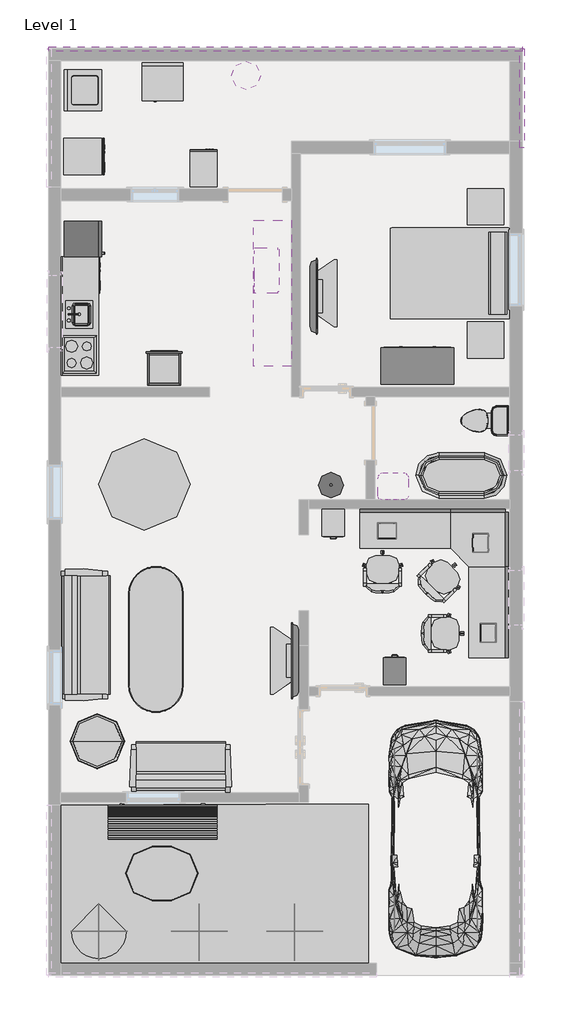
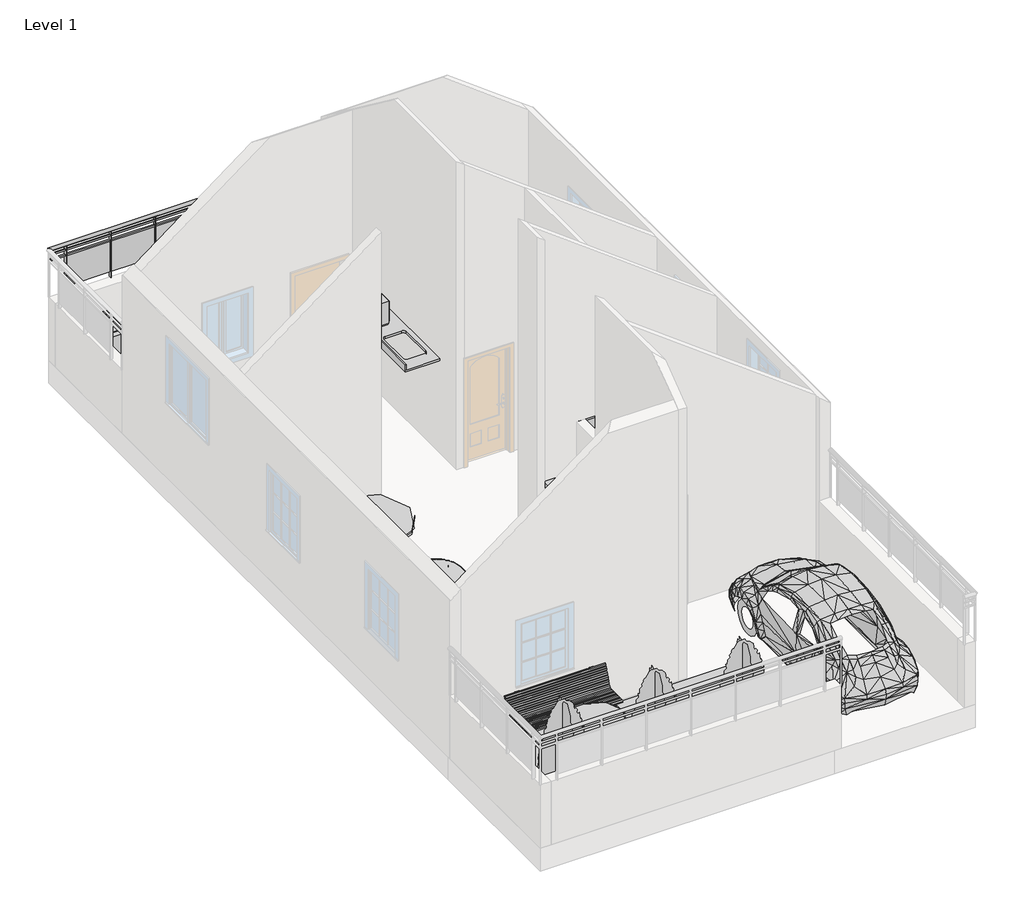
# One storey, part 3 of 3: 22 furniture elements, 15 proxies, 6 flow terminals, 4 geographic elements, 2 railings.
"""IFC4 building model written with IfcOpenShell, lengths in millimetres."""

from ifc_helpers import new_model, si_unit, point, frame, origin, place, context, project, spatial, polyline, ellipse_curve, trimmed, outline, extrude, triangles, transform, mapped, element, save
from ifc_brep_helpers import plane_surface, extruded_surface, advanced_brep
from components import entourage_4c8cfd20, proxy_7e1014cc, proxy_a6faaae8, proxy_45b28599, proxy_19aded4c, proxy_b4d0e45e, kitchenette_medium_kitchenette_medium_844211aa, proxy_8a8d5ab2, proxy_8b8c2dc4, rpc_beetle_rpc_beetle_3ce7ba48, proxy_c523a7b7, proxy_718fa39f, flow_terminal_871c2e40, flow_terminal_d49f872f, flow_terminal_62a433f7, toilet_domestic_3d_toilet_domestic_3d_f7549cf7, toilet_domestic_3d_toilet_domestic_3d_183bbd19, flow_terminal_b374fae2, furniture_e1791683, furniture_bb55ed6b, furniture_b1353b55, chair_executive_chair_executive_8d69e98c, furniture_22cae41e, furniture_c6510c7c, furniture_9fa109b2, furniture_ad7727fe, furniture_aff9b2fb, furniture_fdf74506, tv_stand_tv_stand_6ce107e5, furniture_be1c6672, furniture_e05f6f82, furniture_bbcc68ce, furniture_5bc9ed15, furniture_c80d6d9c, furniture_45e3acac, geographic_element_235d1464, rpc_tree_conifer_chinese_juniper_7_1b9786cd

model = new_model("IFC4")

# Units and contexts
model_context = context("Model", 3, world=origin())
ifc_project = project(units=[si_unit("LENGTHUNIT", "METRE", prefix="MILLI")], contexts=[model_context])

# Site, building, storey
site = spatial("IfcSite", under=ifc_project)
building = spatial("IfcBuilding", under=site)
storey = spatial("IfcBuildingStorey", under=building, Name="Level 1", Elevation=0.0)

# Proxies
placement = place(None, origin())
element("IfcBuildingElementProxy", 1, Name="Building Element Proxy", at=placement, inside=storey, context=model_context, shape_type="Tessellation", body=[
    triangles([(-7981.8122177, -789.0605576, 0.0), (-2825.6124115, -763.6605818, 0.0), (-2825.6124115, -3430.6606544, 0.0), (-7981.8122177, -3430.6606544, 0.0)], [[1, 4, 3], [3, 2, 1]], closed=False),
])
entourage_shape = entourage_4c8cfd20(model_context)
element("IfcBuildingElementProxy", 2, Name="Entourage", at=placement, inside=storey, context=model_context, shape_type="MappedRepresentation", body=[
    mapped(entourage_shape, transform((-793.6124913, 2092.734912, 762.0), x_axis=(0.0, -1.0000000000000004, 0.0), y_axis=(1.0000000000000004, 0.0, 0.0), z_axis=(0.0, 0.0, 1.0))),
])
element("IfcBuildingElementProxy", 3, Name="Entourage", at=placement, inside=storey, context=model_context, shape_type="MappedRepresentation", body=[
    mapped(entourage_shape, transform((-2522.3706258, 3833.7394299, 762.0), x_axis=(1.0000000000000004, 0.0, 0.0), y_axis=(0.0, 1.0000000000000004, 0.0), z_axis=(0.0, 0.0, 1.0))),
])
element("IfcBuildingElementProxy", 4, Name="Entourage", at=placement, inside=storey, context=model_context, shape_type="MappedRepresentation", body=[
    mapped(entourage_shape, transform((-920.6124913, 3598.218512, 762.0), x_axis=(0.0, -1.0000000000000002, 0.0), y_axis=(1.0000000000000002, 0.0, 0.0), z_axis=(0.0, 0.0, 1.0))),
])
proxy_shape = proxy_7e1014cc(model_context)
element("IfcBuildingElementProxy", 5, Name="18\" x 24\" x 34 1/2\"", ObjectType="18\" x 24\" x 34 1/2\"", at=placement, inside=storey, context=model_context, shape_type="MappedRepresentation", body=[
    mapped(proxy_shape, transform((-5288.0950228, 10123.1639947, 0.0), x_axis=(-1.0, 0.0, 0.0), y_axis=(0.0, -1.0, 0.0), z_axis=(0.0, 0.0, 1.0))),
])
proxy_2_shape = proxy_a6faaae8(model_context)
element("IfcBuildingElementProxy", 6, Name="Cook Top-4 Unit2 : 22\" x 20\"", ObjectType="Cook Top-4 Unit2 : 22\" x 20\"", at=placement, inside=storey, context=model_context, shape_type="MappedRepresentation", body=[
    mapped(proxy_2_shape, transform((-7677.0124913, 6745.2144299, 0.0), x_axis=(0.0, 0.9999999999999999, 0.0), y_axis=(-0.9999999999999999, 0.0, 0.0), z_axis=(0.0, 0.0, 1.0))),
])
proxy_3_shape = proxy_45b28599(model_context)
element("IfcBuildingElementProxy", 7, Name="Dishwasher : 24\" x 24\" x 34\"", ObjectType="Dishwasher : 24\" x 24\" x 34\"", at=placement, inside=storey, context=model_context, shape_type="MappedRepresentation", body=[
    mapped(proxy_3_shape, transform((-7385.1629265, 7696.3969614, 0.0), x_axis=(0.0, 0.9999999999999999, 0.0), y_axis=(-0.9999999999999999, 0.0, 0.0), z_axis=(0.0, 0.0, 1.0))),
])
proxy_4_shape = proxy_19aded4c(model_context)
element("IfcBuildingElementProxy", 8, Name="Dishwasher : 24\" x 26 1/4\" x 34 1/2\"", ObjectType="Dishwasher : 24\" x 26 1/4\" x 34 1/2\"", at=placement, inside=storey, context=model_context, shape_type="MappedRepresentation", body=[
    mapped(proxy_4_shape, transform((-7308.9629265, 9674.4219614, 0.0), x_axis=(0.0, 1.0000000000000002, 0.0), y_axis=(-1.0000000000000002, 0.0, 0.0), z_axis=(0.0, 0.0, 1.0))),
])
proxy_5_shape = proxy_b4d0e45e(model_context)
element("IfcBuildingElementProxy", 9, Name="Dryer : 27\" x 25\" x 35\"", ObjectType="Dryer : 27\" x 25\" x 35\"", at=placement, inside=storey, context=model_context, shape_type="MappedRepresentation", body=[
    mapped(proxy_5_shape, transform((-6661.0124913, 10996.5394299, 0.0), x_axis=(1.0000000000000004, 0.0, 0.0), y_axis=(0.0, 1.0000000000000004, 0.0), z_axis=(0.0, 0.0, 1.0))),
])
kitchenette_medium_kitchenette_medium_shape = kitchenette_medium_kitchenette_medium_844211aa(model_context)
element("IfcBuildingElementProxy", 10, Name="Kitchenette - Medium : Kitchenette - Medium", ObjectType="Kitchenette - Medium : Kitchenette - Medium", at=placement, inside=storey, context=model_context, shape_type="MappedRepresentation", body=[
    mapped(kitchenette_medium_kitchenette_medium_shape, transform((-7981.8124913, 7069.376725, 0.0), x_axis=(0.0, 0.9999999999999999, 0.0), y_axis=(-0.9999999999999999, 0.0, 0.0), z_axis=(0.0, 0.0, 1.0))),
])
proxy_6_shape = proxy_8a8d5ab2(model_context)
element("IfcBuildingElementProxy", 11, Name="Microwave : 30\" x 16\" x 18\"", ObjectType="Microwave : 30\" x 16\" x 18\"", at=placement, inside=storey, context=model_context, shape_type="MappedRepresentation", body=[
    mapped(proxy_6_shape, transform((-4180.6819855, 8652.0323072, 914.4), x_axis=(0.0, -1.0000000000000004, 0.0), y_axis=(1.0000000000000004, 0.0, 0.0), z_axis=(0.0, 0.0, 1.0))),
])
proxy_7_shape = proxy_8b8c2dc4(model_context)
element("IfcBuildingElementProxy", 12, Name="Oven Double-Built-in : 21 1/2\" x 39 1/4\" x 21\"", ObjectType="Oven Double-Built-in : 21 1/2\" x 39 1/4\" x 21\"", at=placement, inside=storey, context=model_context, shape_type="MappedRepresentation", body=[
    mapped(proxy_7_shape, transform((-6289.7874186, 6644.9802888, 0.0), x_axis=(-1.0000000000000004, 0.0, 0.0), y_axis=(0.0, -1.0000000000000004, 0.0), z_axis=(0.0, 0.0, 1.0))),
])
rpc_beetle_rpc_beetle_shape = rpc_beetle_rpc_beetle_3ce7ba48(model_context)
element("IfcBuildingElementProxy", 13, Name="RPC Beetle : RPC Beetle", ObjectType="RPC Beetle : RPC Beetle", at=placement, inside=storey, context=model_context, shape_type="MappedRepresentation", body=[
    mapped(rpc_beetle_rpc_beetle_shape, transform((-1708.0124913, -2589.2855701, 0.0), x_axis=(1.0, 0.0, 0.0), y_axis=(0.0, 1.0, 0.0), z_axis=(0.0, 0.0, 1.0))),
])
proxy_8_shape = proxy_c523a7b7(model_context)
element("IfcBuildingElementProxy", 14, Name="Refrigerator : 24\" x 25\" LH", ObjectType="Refrigerator : 24\" x 25\" LH", at=placement, inside=storey, context=model_context, shape_type="MappedRepresentation", body=[
    mapped(proxy_8_shape, transform((-7631.3635198, 8681.9644299, 0.0), x_axis=(0.0, 0.9999999999999999, 0.0), y_axis=(-0.9999999999999999, 0.0, 0.0), z_axis=(0.0, 0.0, 1.0))),
])
proxy_9_shape = proxy_718fa39f(model_context)
element("IfcBuildingElementProxy", 15, Name="Washer : 27\" x 25\" x 35\"", ObjectType="Washer : 27\" x 25\" x 35\"", at=placement, inside=storey, context=model_context, shape_type="MappedRepresentation", body=[
    mapped(proxy_9_shape, transform((-7334.3629265, 10744.3969614, 0.0), x_axis=(0.0, 1.0000000000000027, 0.0), y_axis=(-1.0000000000000027, 0.0, 0.0), z_axis=(0.0, 0.0, 1.0))),
])

# Flow terminals
flow_terminal_shape = flow_terminal_871c2e40(model_context)
element("IfcFlowTerminal", 16, ObjectType="Sink Kitchen-Island : 18\" x 18\"", at=placement, inside=storey, context=model_context, shape_type="MappedRepresentation", body=[
    mapped(flow_terminal_shape, transform((-7674.6670902, 7402.6251893, -14.4), x_axis=(0.0, 0.9999999999999999, 0.0), y_axis=(-0.9999999999999999, 0.0, 0.0), z_axis=(0.0, 0.0, 1.0))),
])
flow_terminal_2_shape = flow_terminal_d49f872f(model_context)
element("IfcFlowTerminal", 17, ObjectType="Sink Vanity-Round : 19\" x 19\"", at=placement, inside=storey, context=model_context, shape_type="MappedRepresentation", body=[
    mapped(flow_terminal_2_shape, transform((-4979.6642319, 11328.3270307, 914.4), x_axis=(1.0, 0.0, 0.0), y_axis=(0.0, 1.0, 0.0), z_axis=(0.0, 0.0, 1.0))),
])
element("IfcFlowTerminal", 18, ObjectType="Sink Vanity-Round : 19\" x 19\"", at=placement, inside=storey, context=model_context, shape_type="MappedRepresentation", body=[
    mapped(flow_terminal_2_shape, transform((-3363.9607507, 4648.8362448, 609.6), x_axis=(-1.0, 0.0, 0.0), y_axis=(0.0, -1.0, 0.0), z_axis=(0.0, 0.0, 1.0))),
])
flow_terminal_3_shape = flow_terminal_62a433f7(model_context)
element("IfcFlowTerminal", 19, ObjectType="Sink Vanity-Square : 20\" x 18\"", at=placement, inside=storey, context=model_context, shape_type="MappedRepresentation", body=[
    mapped(flow_terminal_3_shape, transform((-2403.5232507, 4496.484831, 914.4), x_axis=(-1.0, 0.0, 0.0), y_axis=(0.0, -1.0, 0.0), z_axis=(0.0, 0.0, 1.0))),
])
toilet_domestic_3d_toilet_domestic_3d_shape = toilet_domestic_3d_toilet_domestic_3d_f7549cf7(model_context)
toilet_domestic_3d_toilet_domestic_3d_2_shape = toilet_domestic_3d_toilet_domestic_3d_183bbd19(model_context)
element("IfcFlowTerminal", 20, ObjectType="Toilet-Domestic-3D : Toilet-Domestic-3D", at=placement, inside=storey, context=model_context, shape_type="MappedRepresentation", body=[
    mapped(toilet_domestic_3d_toilet_domestic_3d_shape, transform((-983.5085187, 5640.3144299, 0.0), x_axis=(0.0, -1.0, 0.0), y_axis=(1.0, 0.0, 0.0), z_axis=(0.0, 0.0, 1.0))),
    mapped(toilet_domestic_3d_toilet_domestic_3d_2_shape, transform((-983.5085187, 5640.3144299, 0.0), x_axis=(0.0, -1.0, 0.0), y_axis=(1.0, 0.0, 0.0), z_axis=(0.0, 0.0, 1.0))),
])
flow_terminal_4_shape = flow_terminal_b374fae2(model_context)
element("IfcFlowTerminal", 21, ObjectType="Tub-Free Standing-3D : 30\" x 60\"", at=placement, inside=storey, context=model_context, shape_type="MappedRepresentation", body=[
    mapped(flow_terminal_4_shape, transform((-1276.2124913, 4725.9144299, 0.0), x_axis=(0.0, -1.0000000000000002, 0.0), y_axis=(1.0000000000000002, 0.0, 0.0), z_axis=(0.0, 0.0, 1.0))),
])

# Furniture
furniture_shape = furniture_e1791683(model_context)
element("IfcFurniture", 22, ObjectType="Bed-Standard.0001 : Queen 60\" x 79\"", at=placement, inside=storey, context=model_context, shape_type="MappedRepresentation", body=[
    mapped(furniture_shape, transform((-1421.1174093, 8375.6029545, 0.0), x_axis=(0.0, -1.0, 0.0), y_axis=(1.0, 0.0, 0.0), z_axis=(0.0, 0.0, 1.0))),
])
furniture_2_shape = furniture_bb55ed6b(model_context)
element("IfcFurniture", 23, ObjectType="Cabinet-File 2 Drawer : 15\" x 18\"", at=placement, inside=storey, context=model_context, shape_type="MappedRepresentation", body=[
    mapped(furniture_2_shape, transform((-3294.6160443, 4077.47373, 0.0), x_axis=(1.0, 0.0, 0.0), y_axis=(0.0, 1.0, 0.0), z_axis=(0.0, 0.0, 1.0))),
])
furniture_3_shape = furniture_b1353b55(model_context)
element("IfcFurniture", 24, ObjectType="Cabinet-File 4 Drawer : 15\" x 18\"", at=placement, inside=storey, context=model_context, shape_type="MappedRepresentation", body=[
    mapped(furniture_3_shape, transform((-2521.7089384, 1307.1801298, 0.0), x_axis=(-1.0, 0.0, 0.0), y_axis=(0.0, -1.0, 0.0), z_axis=(0.0, 0.0, 1.0))),
])
chair_executive_chair_executive_shape = chair_executive_chair_executive_8d69e98c(model_context)
element("IfcFurniture", 25, ObjectType="Chair-Executive : Chair-Executive", at=placement, inside=storey, context=model_context, shape_type="MappedRepresentation", body=[
    mapped(chair_executive_chair_executive_shape, transform((-2738.003311, 3103.5935283, 0.0), x_axis=(1.0, 0.0, 0.0), y_axis=(0.0, 1.0, 0.0), z_axis=(0.0, 0.0, 1.0))),
])
element("IfcFurniture", 26, ObjectType="Chair-Executive : Chair-Executive", at=placement, inside=storey, context=model_context, shape_type="MappedRepresentation", body=[
    mapped(chair_executive_chair_executive_shape, transform((-1599.958393, 2222.1302496, 0.0), x_axis=(0.0, -1.0000000000000004, 0.0), y_axis=(1.0000000000000004, 0.0, 0.0), z_axis=(0.0, 0.0, 1.0))),
])
element("IfcFurniture", 27, ObjectType="Chair-Executive : Chair-Executive", at=placement, inside=storey, context=model_context, shape_type="MappedRepresentation", body=[
    mapped(chair_executive_chair_executive_shape, transform((-1730.3328147, 3085.013219, 0.0), x_axis=(0.7071067811865468, -0.7071067811865482, 0.0), y_axis=(0.7071067811865482, 0.7071067811865468, 0.0), z_axis=(0.0, 0.0, 1.0))),
])
furniture_4_shape = furniture_22cae41e(model_context)
element("IfcFurniture", 28, ObjectType="Counter Top w Sink Hole : 24\" Depth", at=placement, inside=storey, context=model_context, shape_type="MappedRepresentation", body=[
    mapped(furniture_4_shape, transform((-4756.0124913, 7755.176725, 914.4), x_axis=(0.0, 1.0, 0.0), y_axis=(-1.0, 0.0, 0.0), z_axis=(0.0, 0.0, 1.0))),
])
furniture_5_shape = furniture_c6510c7c(model_context)
element("IfcFurniture", 29, ObjectType="Counter Top w Sink Hole : 24\" Depth", at=placement, inside=storey, context=model_context, shape_type="MappedRepresentation", body=[
    mapped(furniture_5_shape, transform((-7981.8124913, 7602.776725, -14.4), x_axis=(0.0, 0.9999999999999999, 0.0), y_axis=(-0.9999999999999999, 0.0, 0.0), z_axis=(0.0, 0.0, 1.0))),
])
furniture_6_shape = furniture_9fa109b2(model_context)
element("IfcFurniture", 30, ObjectType="Dresser : 48\" x 72\" x 24\"", at=placement, inside=storey, context=model_context, shape_type="MappedRepresentation", body=[
    mapped(furniture_6_shape, transform((-2282.0057511, 6191.5514758, 0.0), x_axis=(-1.0000000000000004, 0.0, 0.0), y_axis=(0.0, -1.0000000000000004, 0.0), z_axis=(0.0, 0.0, 1.0))),
])
furniture_7_shape = furniture_ad7727fe(model_context)
element("IfcFurniture", 31, ObjectType="Sofa-Pensi : 65\"", at=placement, inside=storey, context=model_context, shape_type="MappedRepresentation", body=[
    mapped(furniture_7_shape, transform((-5696.6062413, 126.224266, 0.0), x_axis=(-1.0, 0.0, 0.0), y_axis=(0.0, -1.0, 0.0), z_axis=(0.0, 0.0, 1.0))),
])
furniture_8_shape = furniture_aff9b2fb(model_context)
element("IfcFurniture", 32, ObjectType="Sofa-Pensi : 84\"", at=placement, inside=storey, context=model_context, shape_type="MappedRepresentation", body=[
    mapped(furniture_8_shape, transform((-7298.3026552, 1780.3081799, 0.0), x_axis=(0.0, 1.0, 0.0), y_axis=(-1.0, 0.0, 0.0), z_axis=(0.0, 0.0, 1.0))),
])
furniture_9_shape = furniture_fdf74506(model_context)
element("IfcFurniture", 33, ObjectType="TV - Flat Screen : 50\"", at=placement, inside=storey, context=model_context, shape_type="MappedRepresentation", body=[
    mapped(furniture_9_shape, transform((-3757.6738677, 7723.883944, 914.4), x_axis=(0.0, 1.0000000000000002, 0.0), y_axis=(-1.0000000000000002, 0.0, 0.0), z_axis=(0.0, 0.0, 1.0))),
])
element("IfcFurniture", 34, ObjectType="TV - Flat Screen : 50\"", at=placement, inside=storey, context=model_context, shape_type="MappedRepresentation", body=[
    mapped(furniture_9_shape, transform((-4052.551115, 1621.6081753, 914.4), x_axis=(0.0, -1.0000000000000007, 0.0), y_axis=(1.0000000000000007, 0.0, 0.0), z_axis=(0.0, 0.0, 1.0))),
])
tv_stand_tv_stand_shape = tv_stand_tv_stand_6ce107e5(model_context)
element("IfcFurniture", 35, ObjectType="TV Stand : TV Stand", at=placement, inside=storey, context=model_context, shape_type="MappedRepresentation", body=[
    mapped(tv_stand_tv_stand_shape, transform((-3816.2124913, 7648.7264278, 0.0), x_axis=(0.0, 1.0, 0.0), y_axis=(-1.0, 0.0, 0.0), z_axis=(0.0, 0.0, 1.0))),
])
element("IfcFurniture", 36, ObjectType="TV Stand : TV Stand", at=placement, inside=storey, context=model_context, shape_type="MappedRepresentation", body=[
    mapped(tv_stand_tv_stand_shape, transform((-4019.4124913, 1752.302432, 0.0), x_axis=(0.0, -1.0000000000000004, 0.0), y_axis=(1.0000000000000004, 0.0, 0.0), z_axis=(0.0, 0.0, 1.0))),
])
furniture_10_shape = furniture_be1c6672(model_context)
element("IfcFurniture", 37, ObjectType="Table-Dining Oval : 36\" x 48\"", at=placement, inside=storey, context=model_context, shape_type="MappedRepresentation", body=[
    mapped(furniture_10_shape, transform((-5889.7477591, -1573.9622094, 0.0), x_axis=(1.0, 0.0, 0.0), y_axis=(0.0, 1.0, 0.0), z_axis=(0.0, 0.0, 1.0))),
])
furniture_11_shape = furniture_e05f6f82(model_context)
element("IfcFurniture", 38, ObjectType="Table-Dining Oval : 36\" x 96\" Laminate Top", at=placement, inside=storey, context=model_context, shape_type="MappedRepresentation", body=[
    mapped(furniture_11_shape, transform((-6748.2575678, 2384.534102, 0.0), x_axis=(0.0, 1.0000000000000002, 0.0), y_axis=(-1.0000000000000002, 0.0, 0.0), z_axis=(0.0, 0.0, 1.0))),
])
furniture_12_shape = furniture_bbcc68ce(model_context)
element("IfcFurniture", 39, ObjectType="Table-Dining Round w Chairs : 60\" Diameter", at=placement, inside=storey, context=model_context, shape_type="MappedRepresentation", body=[
    mapped(furniture_12_shape, transform((-6688.4944585, 4758.3931184, 0.0), x_axis=(1.0, 0.0, 0.0), y_axis=(0.0, 1.0, 0.0), z_axis=(0.0, 0.0, 1.0))),
])
furniture_13_shape = furniture_5bc9ed15(model_context)
element("IfcFurniture", 40, ObjectType="Table-Night Stand : 24\" x 24\" x 30\"", at=placement, inside=storey, context=model_context, shape_type="MappedRepresentation", body=[
    mapped(furniture_13_shape, transform((-1178.3461216, 8913.7394299, 0.0), x_axis=(1.0, 0.0, 0.0), y_axis=(0.0, 1.0, 0.0), z_axis=(0.0, 0.0, 1.0))),
])
element("IfcFurniture", 41, ObjectType="Table-Night Stand : 24\" x 24\" x 30\"", at=placement, inside=storey, context=model_context, shape_type="MappedRepresentation", body=[
    mapped(furniture_13_shape, transform((-1178.3461216, 6681.7144299, 0.0), x_axis=(1.0, 0.0, 0.0), y_axis=(0.0, 1.0, 0.0), z_axis=(0.0, 0.0, 1.0))),
])
furniture_14_shape = furniture_c80d6d9c(model_context)
element("IfcFurniture", 42, ObjectType="Table-Round : 36\" Diameter", at=placement, inside=storey, context=model_context, shape_type="MappedRepresentation", body=[
    mapped(furniture_14_shape, transform((-7372.2124913, 277.7394299, 0.0), x_axis=(1.0, 0.0, 0.0), y_axis=(0.0, 1.0, 0.0), z_axis=(0.0, 0.0, 1.0))),
])
furniture_15_shape = furniture_45e3acac(model_context)
element("IfcFurniture", 43, ObjectType="Work Station Cubicle : 96\" x 96\"", at=placement, inside=storey, context=model_context, shape_type="MappedRepresentation", body=[
    mapped(furniture_15_shape, transform((6.2105163, 4032.2076777, 0.0), x_axis=(0.0, -1.0000000000000004, 0.0), y_axis=(1.0000000000000004, 0.0, 0.0), z_axis=(0.0, 0.0, 1.0))),
])

# Geographic elements
geographic_element_shape = geographic_element_235d1464(model_context)
element("IfcGeographicElement", 44, ObjectType="Park Bench : 72\"", at=placement, inside=storey, context=model_context, shape_type="MappedRepresentation", body=[
    mapped(geographic_element_shape, transform((-6280.0124913, -1043.0605701, 0.0), x_axis=(1.0, 0.0, 0.0), y_axis=(0.0, 1.0, 0.0), z_axis=(0.0, 0.0, 1.0))),
])
rpc_tree_conifer_chinese_juniper_7_shape = rpc_tree_conifer_chinese_juniper_7_1b9786cd(model_context)
element("IfcGeographicElement", 45, ObjectType="RPC Tree - Conifer : Chinese Juniper - 7'", at=placement, inside=storey, context=model_context, shape_type="MappedRepresentation", body=[
    mapped(rpc_tree_conifer_chinese_juniper_7_shape, transform((-7347.0091624, -2897.2605701, 0.0), x_axis=(1.0, 0.0, 0.0), y_axis=(0.0, 1.0, 0.0), z_axis=(0.0, 0.0, 1.0))),
])
element("IfcGeographicElement", 46, ObjectType="RPC Tree - Conifer : Chinese Juniper - 7'", at=placement, inside=storey, context=model_context, shape_type="MappedRepresentation", body=[
    mapped(rpc_tree_conifer_chinese_juniper_7_shape, transform((-5670.6091624, -2897.2605701, 0.0), x_axis=(1.0, 0.0, 0.0), y_axis=(0.0, 1.0, 0.0), z_axis=(0.0, 0.0, 1.0))),
])
element("IfcGeographicElement", 47, ObjectType="RPC Tree - Conifer : Chinese Juniper - 7'", at=placement, inside=storey, context=model_context, shape_type="MappedRepresentation", body=[
    mapped(rpc_tree_conifer_chinese_juniper_7_shape, transform((-4070.4091624, -2897.2605701, 0.0), x_axis=(1.0, 0.0, 0.0), y_axis=(0.0, 1.0, 0.0), z_axis=(0.0, 0.0, 1.0))),
])

# Railings
element("IfcRailing", 48, ObjectType="Glass Panel - Bottom Fill", at=placement, inside=storey, context=model_context, shape_type="SolidModel", body=[
    advanced_brep(
    [(-8185.0124913, 11898.2394299, 2133.6), (-8185.0124913, 11822.0394299, 2133.6), (-260.2124913, 11898.2394299, 2133.6), (-260.2124913, 11822.0394299, 2133.6)],
    [
        (0, 1, ellipse_curve(frame((-8185.0124913, 11860.1394299, 2133.6), z_axis=(-1.0, 0.0, 0.0), x_axis=(0.0, -1.0, 0.0)), 38.1, 28.575)),
        (1, 0, ellipse_curve(frame((-8185.0124913, 11860.1394299, 2133.6), z_axis=(-1.0, 0.0, 0.0), x_axis=(0.0, -1.0, 0.0)), 38.1, 28.575)),
        (2, 3, ellipse_curve(frame((-260.2124913, 11860.1394299, 2133.6), z_axis=(1.0, 0.0, 0.0), x_axis=(0.0, -1.0, 0.0)), 38.1, 28.575)),
        (3, 2, ellipse_curve(frame((-260.2124913, 11860.1394299, 2133.6), z_axis=(1.0, 0.0, 0.0), x_axis=(0.0, -1.0, 0.0)), 38.1, 28.575)),
        (0, 2),
        (3, 1),
    ],
    [
        plane_surface(frame((-8185.0124913, 11860.1394299, 2133.6), z_axis=(-1.0, 0.0, 0.0), x_axis=(0.0, 1.0, 0.0))),
        plane_surface(frame((-260.2124913, 11860.1394299, 2133.6), z_axis=(1.0, 0.0, 0.0), x_axis=(0.0, 1.0, 0.0))),
        extruded_surface(trimmed(ellipse_curve(frame((-260.2124913, 11860.1394299, 2133.6), z_axis=(-1.0, 0.0, 0.0), x_axis=(0.0, -1.0, 0.0)), 38.1, 28.575), [point((-260.2124913, 11898.2394299, 2133.6))], [point((-260.2124913, 11822.0394299, 2133.6))], True, "CARTESIAN"), (-7924.8, 0.0, 0.0), 7924.8),
        extruded_surface(trimmed(ellipse_curve(frame((-260.2124913, 11860.1394299, 2133.6), z_axis=(-1.0, 0.0, 0.0), x_axis=(0.0, -1.0, 0.0)), 38.1, 28.575), [point((-260.2124913, 11822.0394299, 2133.6))], [point((-260.2124913, 11898.2394299, 2133.6))], True, "CARTESIAN"), (-7924.8, 0.0, 0.0), 7924.8),
    ],
    [
        (0, [[1, 2]]),
        (1, [[3, 4]]),
        (2, [[-1, 5, -4, 6]]),
        (3, [[-2, -6, -3, -5]]),
    ],
),
    extrude(outline(polyline([(-8185.0124913, 11847.4394299), (-8185.0124913, 11872.8394299), (-260.2124913, 11872.8394299), (-260.2124913, 11847.4394299), (-8185.0124913, 11847.4394299)])), frame((0.0, 0.0, 2019.3), z_axis=(0.0, 0.0, 1.0), x_axis=(1.0, 0.0, 0.0)), (0.0, 0.0, 1.0), 25.4),
    extrude(outline(polyline([(-8185.0124913, 11847.4394299), (-8185.0124913, 11872.8394299), (-260.2124913, 11872.8394299), (-260.2124913, 11847.4394299), (-8185.0124913, 11847.4394299)])), frame((0.0, 0.0, 1917.7), z_axis=(0.0, 0.0, 1.0), x_axis=(1.0, 0.0, 0.0)), (0.0, 0.0, 1.0), 25.4),
    extrude(outline(polyline([(-571.3624913, 11834.7394299), (-571.3624913, 11885.5394299), (-558.6624913, 11885.5394299), (-558.6624913, 11834.7394299), (-571.3624913, 11834.7394299)])), frame((0.0, 0.0, 1219.2), z_axis=(0.0, 0.0, 1.0), x_axis=(1.0, 0.0, 0.0)), (0.0, 0.0, 1.0), 885.6788223),
    extrude(outline(polyline([(-1377.8124913, 11866.6745869), (-565.0124913, 11866.6745869), (-565.0124913, 11860.3245869), (-1377.8124913, 11860.3245869), (-1377.8124913, 11866.6745869)])), frame((0.0, 0.0, 1320.8), z_axis=(0.0, 0.0, 1.0), x_axis=(1.0, 0.0, 0.0)), (0.0, 0.0, 1.0), 596.9),
    extrude(outline(polyline([(-1384.1624913, 11834.7394299), (-1384.1624913, 11885.5394299), (-1371.4624913, 11885.5394299), (-1371.4624913, 11834.7394299), (-1384.1624913, 11834.7394299)])), frame((0.0, 0.0, 1219.2), z_axis=(0.0, 0.0, 1.0), x_axis=(1.0, 0.0, 0.0)), (0.0, 0.0, 1.0), 885.6788223),
    extrude(outline(polyline([(-2190.6124913, 11866.6745869), (-1377.8124913, 11866.6745869), (-1377.8124913, 11860.3245869), (-2190.6124913, 11860.3245869), (-2190.6124913, 11866.6745869)])), frame((0.0, 0.0, 1320.8), z_axis=(0.0, 0.0, 1.0), x_axis=(1.0, 0.0, 0.0)), (0.0, 0.0, 1.0), 596.9),
    extrude(outline(polyline([(-2196.9624913, 11834.7394299), (-2196.9624913, 11885.5394299), (-2184.2624913, 11885.5394299), (-2184.2624913, 11834.7394299), (-2196.9624913, 11834.7394299)])), frame((0.0, 0.0, 1219.2), z_axis=(0.0, 0.0, 1.0), x_axis=(1.0, 0.0, 0.0)), (0.0, 0.0, 1.0), 885.6788223),
    extrude(outline(polyline([(-3003.4124913, 11866.6745869), (-2190.6124913, 11866.6745869), (-2190.6124913, 11860.3245869), (-3003.4124913, 11860.3245869), (-3003.4124913, 11866.6745869)])), frame((0.0, 0.0, 1320.8), z_axis=(0.0, 0.0, 1.0), x_axis=(1.0, 0.0, 0.0)), (0.0, 0.0, 1.0), 596.9),
    extrude(outline(polyline([(-3009.7624913, 11834.7394299), (-3009.7624913, 11885.5394299), (-2997.0624913, 11885.5394299), (-2997.0624913, 11834.7394299), (-3009.7624913, 11834.7394299)])), frame((0.0, 0.0, 1219.2), z_axis=(0.0, 0.0, 1.0), x_axis=(1.0, 0.0, 0.0)), (0.0, 0.0, 1.0), 885.6788223),
    extrude(outline(polyline([(-3816.2124913, 11866.6745869), (-3003.4124913, 11866.6745869), (-3003.4124913, 11860.3245869), (-3816.2124913, 11860.3245869), (-3816.2124913, 11866.6745869)])), frame((0.0, 0.0, 1320.8), z_axis=(0.0, 0.0, 1.0), x_axis=(1.0, 0.0, 0.0)), (0.0, 0.0, 1.0), 596.9),
    extrude(outline(polyline([(-3822.5624913, 11834.7394299), (-3822.5624913, 11885.5394299), (-3809.8624913, 11885.5394299), (-3809.8624913, 11834.7394299), (-3822.5624913, 11834.7394299)])), frame((0.0, 0.0, 1219.2), z_axis=(0.0, 0.0, 1.0), x_axis=(1.0, 0.0, 0.0)), (0.0, 0.0, 1.0), 885.6788223),
    extrude(outline(polyline([(-4629.0124913, 11866.6745869), (-3816.2124913, 11866.6745869), (-3816.2124913, 11860.3245869), (-4629.0124913, 11860.3245869), (-4629.0124913, 11866.6745869)])), frame((0.0, 0.0, 1320.8), z_axis=(0.0, 0.0, 1.0), x_axis=(1.0, 0.0, 0.0)), (0.0, 0.0, 1.0), 596.9),
    extrude(outline(polyline([(-4635.3624913, 11834.7394299), (-4635.3624913, 11885.5394299), (-4622.6624913, 11885.5394299), (-4622.6624913, 11834.7394299), (-4635.3624913, 11834.7394299)])), frame((0.0, 0.0, 1219.2), z_axis=(0.0, 0.0, 1.0), x_axis=(1.0, 0.0, 0.0)), (0.0, 0.0, 1.0), 885.6788223),
    extrude(outline(polyline([(-5441.8124913, 11866.6745869), (-4629.0124913, 11866.6745869), (-4629.0124913, 11860.3245869), (-5441.8124913, 11860.3245869), (-5441.8124913, 11866.6745869)])), frame((0.0, 0.0, 1320.8), z_axis=(0.0, 0.0, 1.0), x_axis=(1.0, 0.0, 0.0)), (0.0, 0.0, 1.0), 596.9),
    extrude(outline(polyline([(-5448.1624913, 11834.7394299), (-5448.1624913, 11885.5394299), (-5435.4624913, 11885.5394299), (-5435.4624913, 11834.7394299), (-5448.1624913, 11834.7394299)])), frame((0.0, 0.0, 1219.2), z_axis=(0.0, 0.0, 1.0), x_axis=(1.0, 0.0, 0.0)), (0.0, 0.0, 1.0), 885.6788223),
    extrude(outline(polyline([(-6254.6124913, 11866.6745869), (-5441.8124913, 11866.6745869), (-5441.8124913, 11860.3245869), (-6254.6124913, 11860.3245869), (-6254.6124913, 11866.6745869)])), frame((0.0, 0.0, 1320.8), z_axis=(0.0, 0.0, 1.0), x_axis=(1.0, 0.0, 0.0)), (0.0, 0.0, 1.0), 596.9),
    extrude(outline(polyline([(-6260.9624913, 11834.7394299), (-6260.9624913, 11885.5394299), (-6248.2624913, 11885.5394299), (-6248.2624913, 11834.7394299), (-6260.9624913, 11834.7394299)])), frame((0.0, 0.0, 1219.2), z_axis=(0.0, 0.0, 1.0), x_axis=(1.0, 0.0, 0.0)), (0.0, 0.0, 1.0), 885.6788223),
    extrude(outline(polyline([(-7067.4124913, 11866.6745869), (-6254.6124913, 11866.6745869), (-6254.6124913, 11860.3245869), (-7067.4124913, 11860.3245869), (-7067.4124913, 11866.6745869)])), frame((0.0, 0.0, 1320.8), z_axis=(0.0, 0.0, 1.0), x_axis=(1.0, 0.0, 0.0)), (0.0, 0.0, 1.0), 596.9),
    extrude(outline(polyline([(-7073.7624913, 11834.7394299), (-7073.7624913, 11885.5394299), (-7061.0624913, 11885.5394299), (-7061.0624913, 11834.7394299), (-7073.7624913, 11834.7394299)])), frame((0.0, 0.0, 1219.2), z_axis=(0.0, 0.0, 1.0), x_axis=(1.0, 0.0, 0.0)), (0.0, 0.0, 1.0), 885.6788223),
    extrude(outline(polyline([(-7880.2124913, 11866.6745869), (-7067.4124913, 11866.6745869), (-7067.4124913, 11860.3245869), (-7880.2124913, 11860.3245869), (-7880.2124913, 11866.6745869)])), frame((0.0, 0.0, 1320.8), z_axis=(0.0, 0.0, 1.0), x_axis=(1.0, 0.0, 0.0)), (0.0, 0.0, 1.0), 596.9),
    extrude(outline(polyline([(-7886.5624913, 11834.7394299), (-7886.5624913, 11885.5394299), (-7873.8624913, 11885.5394299), (-7873.8624913, 11834.7394299), (-7886.5624913, 11834.7394299)])), frame((0.0, 0.0, 1219.2), z_axis=(0.0, 0.0, 1.0), x_axis=(1.0, 0.0, 0.0)), (0.0, 0.0, 1.0), 885.6788223),
    extrude(outline(polyline([(-272.9124913, 11850.6144299), (-272.9124913, 11869.6644299), (-253.8624913, 11869.6644299), (-253.8624913, 11850.6144299), (-272.9124913, 11850.6144299)])), frame((0.0, 0.0, 1219.2), z_axis=(0.0, 0.0, 1.0), x_axis=(1.0, 0.0, 0.0)), (0.0, 0.0, 1.0), 885.6788223),
    extrude(outline(polyline([(-8191.3624913, 11850.6144299), (-8191.3624913, 11869.6644299), (-8172.3124913, 11869.6644299), (-8172.3124913, 11850.6144299), (-8191.3624913, 11850.6144299)])), frame((0.0, 0.0, 1219.2), z_axis=(0.0, 0.0, 1.0), x_axis=(1.0, 0.0, 0.0)), (0.0, 0.0, 1.0), 885.6788223),
])
element("IfcRailing", 49, ObjectType="Glass Panel - Bottom Fill", at=placement, inside=storey, context=model_context, shape_type="SolidModel", body=[
    advanced_brep(
    [(-298.3124913, 10209.1394299, 2133.6), (-222.1124913, 10209.1394299, 2133.6), (-298.3124913, 11860.1394299, 2133.6), (-222.1124913, 11860.1394299, 2133.6)],
    [
        (0, 1, ellipse_curve(frame((-260.2124913, 10209.1394299, 2133.6), z_axis=(0.0, -1.0, 0.0), x_axis=(1.0, 0.0, 0.0)), 38.1, 28.575)),
        (1, 0, ellipse_curve(frame((-260.2124913, 10209.1394299, 2133.6), z_axis=(0.0, -1.0, 0.0), x_axis=(1.0, 0.0, 0.0)), 38.1, 28.575)),
        (2, 3, ellipse_curve(frame((-260.2124913, 11860.1394299, 2133.6), z_axis=(0.0, 1.0, 0.0), x_axis=(1.0, 0.0, 0.0)), 38.1, 28.575)),
        (3, 2, ellipse_curve(frame((-260.2124913, 11860.1394299, 2133.6), z_axis=(0.0, 1.0, 0.0), x_axis=(1.0, 0.0, 0.0)), 38.1, 28.575)),
        (0, 2),
        (3, 1),
    ],
    [
        plane_surface(frame((-260.2124913, 10209.1394299, 2133.6), z_axis=(0.0, -1.0, 0.0), x_axis=(0.0, 0.0, 1.0))),
        plane_surface(frame((-260.2124913, 11860.1394299, 2133.6), z_axis=(0.0, 1.0, 0.0), x_axis=(0.0, 0.0, 1.0))),
        extruded_surface(trimmed(ellipse_curve(frame((-260.2124913, 11860.1394299, 2133.6), z_axis=(0.0, -1.0, 0.0), x_axis=(1.0, 0.0, 0.0)), 38.1, 28.575), [point((-298.3124913, 11860.1394299, 2133.6))], [point((-222.1124913, 11860.1394299, 2133.6))], True, "CARTESIAN"), (0.0, -1651.0, 0.0), 1651.0),
        extruded_surface(trimmed(ellipse_curve(frame((-260.2124913, 11860.1394299, 2133.6), z_axis=(0.0, -1.0, 0.0), x_axis=(1.0, 0.0, 0.0)), 38.1, 28.575), [point((-222.1124913, 11860.1394299, 2133.6))], [point((-298.3124913, 11860.1394299, 2133.6))], True, "CARTESIAN"), (0.0, -1651.0, 0.0), 1651.0),
    ],
    [
        (0, [[1, 2]]),
        (1, [[3, 4]]),
        (2, [[-1, 5, -4, 6]]),
        (3, [[-2, -6, -3, -5]]),
    ],
),
    extrude(outline(polyline([(-247.5124913, 10209.1394299), (-272.9124913, 10209.1394299), (-272.9124913, 11860.1394299), (-247.5124913, 11860.1394299), (-247.5124913, 10209.1394299)])), frame((0.0, 0.0, 2019.3), z_axis=(0.0, 0.0, 1.0), x_axis=(1.0, 0.0, 0.0)), (0.0, 0.0, 1.0), 25.4),
    extrude(outline(polyline([(-247.5124913, 10209.1394299), (-272.9124913, 10209.1394299), (-272.9124913, 11860.1394299), (-247.5124913, 11860.1394299), (-247.5124913, 10209.1394299)])), frame((0.0, 0.0, 1917.7), z_axis=(0.0, 0.0, 1.0), x_axis=(1.0, 0.0, 0.0)), (0.0, 0.0, 1.0), 25.4),
    extrude(outline(polyline([(-234.8124913, 11841.0894299), (-285.6124913, 11841.0894299), (-285.6124913, 11853.7894299), (-234.8124913, 11853.7894299), (-234.8124913, 11841.0894299)])), frame((0.0, 0.0, 1219.2), z_axis=(0.0, 0.0, 1.0), x_axis=(1.0, 0.0, 0.0)), (0.0, 0.0, 1.0), 885.6788223),
    extrude(outline(polyline([(-266.7476483, 11034.6394299), (-266.7476483, 11847.4394299), (-260.3976483, 11847.4394299), (-260.3976483, 11034.6394299), (-266.7476483, 11034.6394299)])), frame((0.0, 0.0, 1320.8), z_axis=(0.0, 0.0, 1.0), x_axis=(1.0, 0.0, 0.0)), (0.0, 0.0, 1.0), 596.9),
    extrude(outline(polyline([(-234.8124913, 11028.2894299), (-285.6124913, 11028.2894299), (-285.6124913, 11040.9894299), (-234.8124913, 11040.9894299), (-234.8124913, 11028.2894299)])), frame((0.0, 0.0, 1219.2), z_axis=(0.0, 0.0, 1.0), x_axis=(1.0, 0.0, 0.0)), (0.0, 0.0, 1.0), 885.6788223),
    extrude(outline(polyline([(-266.7476483, 10221.8394299), (-266.7476483, 11034.6394299), (-260.3976483, 11034.6394299), (-260.3976483, 10221.8394299), (-266.7476483, 10221.8394299)])), frame((0.0, 0.0, 1320.8), z_axis=(0.0, 0.0, 1.0), x_axis=(1.0, 0.0, 0.0)), (0.0, 0.0, 1.0), 596.9),
    extrude(outline(polyline([(-234.8124913, 10215.4894299), (-285.6124913, 10215.4894299), (-285.6124913, 10228.1894299), (-234.8124913, 10228.1894299), (-234.8124913, 10215.4894299)])), frame((0.0, 0.0, 1219.2), z_axis=(0.0, 0.0, 1.0), x_axis=(1.0, 0.0, 0.0)), (0.0, 0.0, 1.0), 885.6788223),
    extrude(outline(polyline([(-250.6874913, 11847.4394299), (-269.7374913, 11847.4394299), (-269.7374913, 11866.4894299), (-250.6874913, 11866.4894299), (-250.6874913, 11847.4394299)])), frame((0.0, 0.0, 1219.2), z_axis=(0.0, 0.0, 1.0), x_axis=(1.0, 0.0, 0.0)), (0.0, 0.0, 1.0), 885.6788223),
    extrude(outline(polyline([(-250.6874913, 10202.7894299), (-269.7374913, 10202.7894299), (-269.7374913, 10221.8394299), (-250.6874913, 10221.8394299), (-250.6874913, 10202.7894299)])), frame((0.0, 0.0, 1219.2), z_axis=(0.0, 0.0, 1.0), x_axis=(1.0, 0.0, 0.0)), (0.0, 0.0, 1.0), 885.6788223),
])

save(model, "model.ifc")

# Revit data of these elements
# Type
#   built-in parameter 1005195 = "RPC-16-N04H-AQSP-D1N4-43SU-6GKQ-C3KU-1C"
#   Height = 0
# Type "18\" x 24\" x 34 1/2\""
#   Label = "T"
#   Assembly Code = "E1090400"
#   Depth = 2' - 0"
#   Height = 2' - 10 1/2"
#   Width = 1' - 6"
#   Panel Face Material = Plastic, Opaque Black
#   Trach Compact. Material = Steel, Paint Finish, Ivory, Matte
#   Default Elevation = 0
# Type "Cook Top-4 Unit2 : 22\" x 20\""
#   Depth = 1' - 8"
#   Width = 1' - 10"
#   Burner Material = Steel, Chrome Plated
#   Cooktop Material = Steel, Polished
#   Default Elevation = 0
#   Assembly Code = ""
# Type "Dishwasher : 24\" x 24\" x 34\""
#   Label = "DW"
#   Assembly Code = "E1090400"
#   Depth = 2' - 0"
#   Height = 2' - 10"
#   Width = 2' - 0"
#   Dishwasher Material = Steel, Paint Finish, Ivory, Glossy
#   Panel Face Material = Plastic, Opaque Black
#   Default Elevation = 0
# Type "Dishwasher : 24\" x 26 1/4\" x 34 1/2\""
#   Label = "DW"
#   Assembly Code = "E1090400"
#   Depth = 2' - 2 1/4"
#   Height = 2' - 10 1/2"
#   Width = 2' - 0"
#   Dishwasher Material = Steel, Paint Finish, Ivory, Glossy
#   Panel Face Material = Plastic, Opaque Black
#   Default Elevation = 0
# Type "Dryer : 27\" x 25\" x 35\""
#   Label = "D"
#   Assembly Code = "E1090400"
#   Depth = 2' - 1"
#   Height = 2' - 11"
#   Width = 2' - 3"
#   Dryer Material = Steel, Paint Finish, Ivory, Glossy
#   Default Elevation = 0
# Type "Kitchenette - Medium : Kitchenette - Medium"
#   Assembly Code = "E1090400"
#   Counter Length = 6' - 6"
#   Cabinet Width = 4' - 6"
#   Cabinet Height = 2' - 10 1/2"
#   Cabinet Depth = 2' - 0"
#   Toe Depth = 0' - 3"
#   Toe Height = 0' - 3 1/2"
#   Cabinet Material = Cabinets
#   Door/Drawer Material = Cabinets
#   Handle Material = Cabinets - Handles
#   Default Elevation = 0
# Type "Microwave : 30\" x 16\" x 18\""
#   Assembly Code = "E1090400"
#   Depth = 1' - 4"
#   Height = 1' - 6"
#   Width = 2' - 6"
#   Microwave Material = Laminate, Ivory, Matte
#   Default Elevation = 0
# Type "Oven Double-Built-in : 21 1/2\" x 39 1/4\" x 21\""
#   Label = "OVEN"
#   Assembly Code = "E1090400"
#   Depth = 1' - 9"
#   Height = 3' - 3 1/4"
#   Width = 1' - 9 1/2"
#   Oven Material = Metal - Stainless Steel, Polished
#   Default Elevation = 0
# Type "RPC Beetle : RPC Beetle"
#   built-in parameter 1005195 = "RPC-16-0U6E-L4EG-ENH1-J3KF-SVEL-0TX4-C0"
#   Height = 0
# Type "Refrigerator : 24\" x 25\" LH"
#   Label = "REF."
#   Assembly Code = "E1090400"
#   Depth = 2' - 0 3/4"
#   Handle = 0' - 1 1/2"
#   Height = 5' - 3 1/2"
#   Rear Clearance = 0' - 2"
#   Top Door Height = 1' - 8"
#   Width = 1' - 11 1/2"
#   Material = Steel, Paint Finish, Ivory, Glossy
#   Default Elevation = 0
# Type "Washer : 27\" x 25\" x 35\""
#   Label = "W"
#   Assembly Code = "E1090400"
#   Depth = 2' - 1"
#   Height = 2' - 11"
#   Width = 2' - 3"
#   Washer Material = Steel, Paint Finish, Ivory, Matte
#   Default Elevation = 0
# Type "Sink Kitchen-Island : 18\" x 18\""
#   Assembly Code = "D2010410"
#   Counter Height = 3' - 0"
#   Depth = 1' - 6"
#   Width = 1' - 6"
#   Faucet Material = Steel, Polished
#   Sink Material = Steel, Polished
#   Default Elevation = 0
# Type "Sink Vanity-Round : 19\" x 19\""
#   Assembly Code = "D2010400"
#   Top Of Counter = 2' - 7"
#   Basin Material = Porcelain, Linen
#   Faucet Material = Steel, Polished
#   Default Elevation = 0
# Type "Sink Vanity-Square : 20\" x 18\""
#   Assembly Code = "D2010400"
#   Counter Height = 2' - 7"
#   Depth = 1' - 6"
#   Width = 1' - 8"
#   Basin Material = Porcelain, Linen
#   Faucet Material = Steel, Polished
#   Default Elevation = 0
# Type "Toilet-Domestic-3D : Toilet-Domestic-3D"
#   Assembly Code = "D2010110"
#   Toilet - Bowl/Basin Material = Porcelain, Linen
#   Toilet - Seat Material = Laminate, Linen, Matte
#   Default Elevation = 0
# Type "Tub-Free Standing-3D : 30\" x 60\""
#   Assembly Code = "D2010110"
#   Height = 1' - 6"
#   Length = 5' - 0"
#   Width = 2' - 6"
#   Tub Material = Porcelain, Ivory
#   Default Elevation = 0
# Type "Bed-Standard.0001 : Queen 60\" x 79\""
#   Assembly Code = "E2020200"
#   Length = 6' - 7"
#   Width = 5' - 0"
#   Leg Material = Steel, Chrome Plated
#   Mattress Material = Linen, White
#   Default Elevation = 0
# Type "Cabinet-File 2 Drawer : 15\" x 18\""
#   Assembly Code = "E2020200"
#   Depth = 1' - 6"
#   Height = 2' - 5"
#   Width = 1' - 3"
#   Cabinet Material = Steel, Paint Finish, Ivory, Glossy
#   Handle Material = Steel, Chrome Plated
#   Default Elevation = 0
# Type "Cabinet-File 4 Drawer : 15\" x 18\""
#   Assembly Code = "E2020200"
#   Depth = 1' - 6"
#   Height = 4' - 4"
#   Width = 1' - 3"
#   Cabinet Material = Steel, Paint Finish, Ivory, Glossy
#   Handle Material = Steel, Chrome Plated
#   Default Elevation = 0
# Type "Chair-Executive : Chair-Executive"
#   Assembly Code = "E2020200"
#   Base/Arms Material = Plastic, Opaque Black
#   Casters Material = Plastic, Opaque Black
#   Seat/Back Material = Textile - Slate Blue
#   Default Elevation = 0
# Type "Counter Top w Sink Hole : 24\" Depth"
#   Assembly Code = "C1030400"
#   Counter Thickness = 0' - 1 1/2"
#   Depth = 2' - 1"
#   Height = 3' - 0"
#   Length [instance default] = 8' - 0"
#   Sink Location [instance default] = 2' - 0"
#   Sink Location To Wall [instance default] = 0' - 6"
#   Sink Opening Depth [instance default] = 1' - 3"
#   Sink Opening Width [instance default] = 2' - 3"
#   Counter Top Material = none
#   Default Elevation = 0
# Type "Dresser : 48\" x 72\" x 24\""
#   Assembly Code = "E2020200"
#   Depth = 2' - 0"
#   Height = 6' - 0"
#   Width = 4' - 0"
#   Dresser Material = Laminate - Ivory, Glossy
#   Drawer Material = Laminate, Ivory, Matte
#   Knob Material = Cherry
#   Default Elevation = 0
# Type "Sofa-Pensi : 65\""
#   Assembly Code = "E2020200"
#   Length = 5' - 5"
#   Frame Material = Cherry
#   Seat Material = Linen, Beige
#   Feet Material = Steel, Chrome Plated
#   Default Elevation = 0
# Type "Sofa-Pensi : 84\""
#   Assembly Code = "E2020200"
#   Length = 7' - 0"
#   Frame Material = Cherry
#   Seat Material = Linen, Beige
#   Feet Material = Steel, Chrome Plated
#   Default Elevation = 0
# Type "TV - Flat Screen : 50\""
#   SinAng = 0' - 0.0193"
#   L = 3' - 7.57782"
#   H = 2' - 0.51477"
#   Thickness = 0' - 4.33071"
#   Diagonal = 4' - 2"
#   CosAng = 0' - 0.03431"
#   Stand [instance default] = yes
#   Default Elevation = 0
# Type "TV Stand : TV Stand"
#   Depth = 1' - 6"
#   Width = 3' - 8"
#   Height = 1' - 7 1/2"
#   Finish = Melamine - Gray
#   Default Elevation = 0
# Type "Table-Dining Oval : 36\" x 48\""
#   Assembly Code = "E2020200"
#   Length = 4' - 0"
#   Width = 3' - 0"
#   Base Material = Steel, Chrome Plated
#   Top Material = Glass - Clear, Grey
#   Default Elevation = 0
#   Description = (empty or 0)
# Type "Table-Dining Oval : 36\" x 96\" Laminate Top"
#   Assembly Code = "E2020200"
#   Length = 8' - 0"
#   Width = 3' - 0"
#   Base Material = Metal - Bronze, Light Brush
#   Top Material = Laminate, Ivory, Matte
#   Default Elevation = 0
#   Description = (empty or 0)
# Type "Table-Dining Round w Chairs : 60\" Diameter"
#   Assembly Code = "E2020200"
#   Radius = 2' - 6"
#   Diameter = 5' - 0"
#   Height = 2' - 6"
#   Chairs = 6
#   Base Material = Pine
#   Top Material = Laminate, Linen, Matte
#   Default Elevation = 0
# Type "Table-Night Stand : 24\" x 24\" x 30\""
#   Assembly Code = "E2020200"
#   Depth = 2' - 0"
#   Height = 2' - 6"
#   Width = 2' - 0"
#   Base Material = Birch
#   Top Material = Laminate, Ivory, Matte
#   Default Elevation = 0
# Type "Table-Round : 36\" Diameter"
#   Assembly Code = "E2020200"
#   Base Radius = 0' - 10"
#   Height = 2' - 6"
#   Radius = 1' - 6"
#   Base Material = Steel, Chrome Plated
#   Top Material = Birch
#   Default Elevation = 0
# Type "Work Station Cubicle : 96\" x 96\""
#   Assembly Code = "E2020"
#   Desktop Height = 2' - 6"
#   Desktop1 Width = 2' - 0"
#   Desktop2 Width = 2' - 0"
#   Panel Height = 5' - 6"
#   Panel1 Length = 5' - 0"
#   Panel2 Length = 5' - 0"
#   Cube Panel Material = Textile - Light Gray
#   Work Top Material = Laminate, Ivory, Matte
#   Default Elevation = 0
# Type "Park Bench : 72\""
#   Length = 6' - 0"
#   Seat Material = Wood - Teak
#   Frame Material = Steel, Paint Finish, Dark Gray, Matte
# Type "RPC Tree - Conifer : Chinese Juniper - 7'"
#   built-in parameter 1005198 = "{2, 15},{39, RPC-16-FUM3-UUQ0-UBF0-N000-ST1L-LVER-AU},{1, 0},{1, 0},{2, 13},{1, 8},{5, Color},{1, 0},{1, 0},{3, 0.8},{3, 0.8},{3, 0.8},{1, 8},{7, BBoxMin},{1, 0},{1, 0},{1, 0},{1, 0},{1, 0},{1, 8},{7, BBoxMax},{1, 0},{1, 0},{1, 0},{1, 0},{1, 0},{2, 11},{9, RPCTypeId},{1, 0},{1, 0},{39, RPC-16-FUM3-UUQ0-UBF0-N000-ST1L-LVER-AU},{1, 6},{14, RPCPlantHeight},{1, 0},{1, 0},{1, 7},{2, 11},{7, keyword},{1, 0},{1, 0},{34, :RPCs:Trees [General]:Geometry:RPC},{2, 11},{8, category},{1, 0},{1, 0},{15, Trees [General]},{2, 11},{12, LocalizedUID},{1, 0},{1, 0},{15, Chinese Juniper},{2, 14},{6, Height},{1, 0},{1, 0},{1, 7},{1, 2},{16, Cast Reflections},{1, 0},{1, 0},{1, 0},{1, 2},{12, Cast Shadows},{1, 0},{1, 0},{1, 1},{1, 2},{9, Lock View},{1, 0},{1, 0},{1, 0},{1, 4},{5, ViewC},{1, 0},{1, 0},{1, 0},{21, assetlibrary_base.fbx},{1, 5},"
#   built-in parameter 1005195 = "RPC-16-FUM3-UUQ0-UBF0-N000-ST1L-LVER-AU"
#   Type Comments = "Chinese Juniper"
#   Assembly Code = "G2050500"
#   Height = 7' - 0"
#   Description = (empty or 0)
#   Default Elevation = 0
# Type "Glass Panel - Bottom Fill"
#   Assembly Code = "C2010400"
#   built-in parameter 1008612 = 0.0416667 (stored number, unit not read)
#   built-in parameter 1008611 = 0.0416667 (stored number, unit not read)
#   built-in parameter 1008609 = 0.333333 (stored number, unit not read)
#   built-in parameter 1008604 = 0.166667 (stored number, unit not read)
#   built-in parameter 1008603 = 0.166667 (stored number, unit not read)
#   Railing Height = 3' - 0"
#   built-in parameter 1008630 = 2
#   built-in parameter 1008610 = 2
#   built-in parameter 1008618 = Baluster - Square : 3/4"
# Element 1 (IfcBuildingElementProxy)
#   Material = Default Mass Zone
#   Phase Created = New Construction
# Elements 2, 3, 4 (IfcBuildingElementProxy)
#   Phase Created = New Construction
# Element 5 (IfcBuildingElementProxy, "18\" x 24\" x 34 1/2\"")
#   Phase Created = New Construction
#   Materials on its faces: "Steel, Paint Finish, Ivory, Matte", "Plastic, Opaque Black"
# Element 6 (IfcBuildingElementProxy, "Cook Top-4 Unit2 : 22\" x 20\"")
#   Phase Created = New Construction
#   Materials on its faces: "Steel, Chrome Plated", "Steel, Polished"
# Element 7 (IfcBuildingElementProxy, "Dishwasher : 24\" x 24\" x 34\"")
#   Phase Created = New Construction
#   Materials on its faces: "Steel, Paint Finish, Ivory, Glossy", "Plastic, Opaque Black"
# Element 8 (IfcBuildingElementProxy, "Dishwasher : 24\" x 26 1/4\" x 34 1/2\"")
#   Phase Created = New Construction
#   Materials on its faces: "Steel, Paint Finish, Ivory, Glossy", "Plastic, Opaque Black"
# Element 9 (IfcBuildingElementProxy, "Dryer : 27\" x 25\" x 35\"")
#   Phase Created = New Construction
#   Materials on its faces: "Steel, Paint Finish, Ivory, Glossy"
# Element 10 (IfcBuildingElementProxy, "Kitchenette - Medium : Kitchenette - Medium")
#   Phase Created = New Construction
#   Materials on its faces: "Cabinets", "Cabinets - Handles"
# Element 11 (IfcBuildingElementProxy, "Microwave : 30\" x 16\" x 18\"")
#   Phase Created = New Construction
#   Materials on its faces: "Laminate, Ivory, Matte", "Glass"
# Element 12 (IfcBuildingElementProxy, "Oven Double-Built-in : 21 1/2\" x 39 1/4\" x 21\"")
#   Phase Created = New Construction
#   Materials on its faces: "Steel", "Metal - Stainless Steel, Polished", "Glass"
# Element 13 (IfcBuildingElementProxy, "RPC Beetle : RPC Beetle")
#   Phase Created = New Construction
# Element 14 (IfcBuildingElementProxy, "Refrigerator : 24\" x 25\" LH")
#   Phase Created = New Construction
#   Materials on its faces: "Steel, Paint Finish, Ivory, Glossy", "Steel, Chrome Plated"
# Element 15 (IfcBuildingElementProxy, "Washer : 27\" x 25\" x 35\"")
#   Phase Created = New Construction
#   Materials on its faces: "Steel, Paint Finish, Ivory, Matte"
# Element 16 (IfcFlowTerminal, "Sink Kitchen-Island : 18\" x 18\"")
#   Mark = "4"
#   Phase Created = New Construction
#   Materials on its faces: "Steel, Polished"
# Element 17 (IfcFlowTerminal, "Sink Vanity-Round : 19\" x 19\"")
#   Mark = "5"
#   Phase Created = New Construction
#   Materials on its faces: "Porcelain, Linen", "Steel, Polished"
# Element 18 (IfcFlowTerminal, "Sink Vanity-Round : 19\" x 19\"")
#   Mark = "6"
#   Phase Created = New Construction
#   Materials on its faces: "Porcelain, Linen", "Steel, Polished"
# Element 19 (IfcFlowTerminal, "Sink Vanity-Square : 20\" x 18\"")
#   Mark = "3"
#   Phase Created = New Construction
#   Materials on its faces: "Porcelain, Linen", "Steel, Polished"
# Element 20 (IfcFlowTerminal, "Toilet-Domestic-3D : Toilet-Domestic-3D")
#   Mark = "2"
#   Phase Created = New Construction
#   Materials on its faces: "Porcelain, Linen", "Laminate, Linen, Matte"
# Element 21 (IfcFlowTerminal, "Tub-Free Standing-3D : 30\" x 60\"")
#   Mark = "1"
#   Phase Created = New Construction
#   Materials on its faces: "Porcelain, Ivory"
# Element 22 (IfcFurniture, "Bed-Standard.0001 : Queen 60\" x 79\"")
#   Phase Created = New Construction
#   Materials on its faces: "Linen, White", "Steel, Chrome Plated"
# Element 23 (IfcFurniture, "Cabinet-File 2 Drawer : 15\" x 18\"")
#   Phase Created = New Construction
#   Materials on its faces: "Steel, Chrome Plated", "Steel, Paint Finish, Ivory, Glossy"
# Element 24 (IfcFurniture, "Cabinet-File 4 Drawer : 15\" x 18\"")
#   Phase Created = New Construction
#   Materials on its faces: "Steel, Chrome Plated", "Steel, Paint Finish, Ivory, Glossy"
# Elements 25, 26, 27 (IfcFurniture, "Chair-Executive : Chair-Executive")
#   Phase Created = New Construction
#   Materials on its faces: "Plastic, Opaque Black", "Textile - Slate Blue"
# Element 28 (IfcFurniture, "Counter Top w Sink Hole : 24\" Depth")
#   Sink Opening Width = 2' - 3"
#   Sink Opening Depth = 1' - 3"
#   Sink Location To Wall = 0' - 6"
#   Sink Location = 2' - 0"
#   Length = 8' - 0"
#   Phase Created = New Construction
#   Materials on its faces: "Counter Top"
# Element 29 (IfcFurniture, "Counter Top w Sink Hole : 24\" Depth")
#   Sink Opening Depth = 1' - 2"
#   Sink Location To Wall = 0' - 6"
#   Length = 6' - 6"
#   Sink Location = 3' - 4"
#   Sink Opening Width = 1' - 4"
#   Phase Created = New Construction
#   Materials on its faces: "Counter Top"
# Element 30 (IfcFurniture, "Dresser : 48\" x 72\" x 24\"")
#   Phase Created = New Construction
#   Materials on its faces: "Laminate, Ivory, Matte", "Cherry", "Laminate - Ivory, Glossy"
# Element 31 (IfcFurniture, "Sofa-Pensi : 65\"")
#   Phase Created = New Construction
#   Materials on its faces: "Cherry", "Linen, Beige", "Steel, Chrome Plated"
# Element 32 (IfcFurniture, "Sofa-Pensi : 84\"")
#   Phase Created = New Construction
#   Materials on its faces: "Cherry", "Linen, Beige", "Steel, Chrome Plated"
# Elements 33, 34 (IfcFurniture, "TV - Flat Screen : 50\"")
#   Stand = yes
#   Phase Created = New Construction
#   Materials on its faces: "TV - Black", "TV - Glass", "TV - Screen"
# Elements 35, 36 (IfcFurniture, "TV Stand : TV Stand")
#   Phase Created = New Construction
#   Materials on its faces: "Melamine - Gray", "Glass - Shelves"
# Element 37 (IfcFurniture, "Table-Dining Oval : 36\" x 48\"")
#   Phase Created = New Construction
#   Materials on its faces: "Steel, Chrome Plated", "Glass - Clear, Grey"
# Element 38 (IfcFurniture, "Table-Dining Oval : 36\" x 96\" Laminate Top")
#   Phase Created = New Construction
#   Materials on its faces: "Metal - Bronze, Light Brush", "Glass - Clear, Grey", "Laminate, Ivory, Matte"
# Element 39 (IfcFurniture, "Table-Dining Round w Chairs : 60\" Diameter")
#   Phase Created = New Construction
#   Materials on its faces: "Pine", "Laminate, Linen, Matte"
# Elements 40, 41 (IfcFurniture, "Table-Night Stand : 24\" x 24\" x 30\"")
#   Phase Created = New Construction
#   Materials on its faces: "Birch", "Laminate, Ivory, Matte"
# Element 42 (IfcFurniture, "Table-Round : 36\" Diameter")
#   Phase Created = New Construction
#   Materials on its faces: "Steel, Chrome Plated", "Birch"
# Element 43 (IfcFurniture, "Work Station Cubicle : 96\" x 96\"")
#   Phase Created = New Construction
#   Materials on its faces: "Textile - Light Gray", "Laminate, Ivory, Matte"
# Element 44 (IfcGeographicElement, "Park Bench : 72\"")
#   Phase Created = New Construction
#   Materials on its faces: "Wood - Teak", "Steel, Paint Finish, Dark Gray, Matte"
# Elements 45, 46, 47 (IfcGeographicElement, "RPC Tree - Conifer : Chinese Juniper - 7'")
#   Phase Created = New Construction
# Elements 48, 49 (IfcRailing, "Glass Panel - Bottom Fill")
#   built-in parameter 1008621 = 4 (stored number, unit not read)
#   Phase Created = New Construction
#   Materials on its faces: "Glass"
# Materials
#   "Plastic, Opaque Black": class "Plastic", colour RGB 0 0 0, transparency 0.7, Description = "Plastic, generic, opaque black", Cost = 0
#   "Steel, Paint Finish, Ivory, Matte": class "Metal", colour RGB 247 247 239, transparency 0, Description = "Steel, paint finish, ivory, matte", Cost = 0
#   "Steel, Chrome Plated": class "Metal", colour RGB 17 17 17, transparency 0, Description = "Chromiuim plated steel", Cost = 0
#   "Steel, Polished": class "Metal", colour RGB 57 57 57, transparency 0, Description = "Polished steel", Cost = 0
#   "Steel, Paint Finish, Ivory, Glossy": class "Metal", colour RGB 247 247 239, transparency 0, Description = "Steel, paint finish, ivory, glossy", Cost = 0
#   "Cabinets": colour RGB 249 249 249, transparency 0
#   "Cabinets - Handles": class "Metal", colour RGB 57 57 57, transparency 0
#   "Laminate, Ivory, Matte": class "Plastic", colour RGB 247 247 239, transparency 0, Description = "Plastic Laminate - Ivory, Matte", Cost = 0
#   "Metal - Stainless Steel, Polished": class "Metal", colour RGB 216 216 216, transparency 0
#   "Porcelain, Linen": class "Ceramic", colour RGB 249 239 230, transparency 0, Description = "Porcelain, linen", Cost = 0
#   "Laminate, Linen, Matte": class "Plastic", colour RGB 249 239 230, transparency 0, Description = "Plastic Laminate - Linen, Matte", Cost = 0
#   "Porcelain, Ivory": class "Ceramic", colour RGB 247 247 239, transparency 0, Description = "Porcelain, ivory", Cost = 0
#   "Linen, White": class "Textile", colour RGB 247 247 239, transparency 0, Description = "Linen, white", Cost = 0
#   "Textile - Slate Blue": class "Fabric", colour RGB 98 102 118, transparency 0
#   "Laminate - Ivory, Glossy": colour RGB 247 247 239, transparency 0
#   "Cherry": class "Wood", colour RGB 226 177 128, transparency 0, Description = "Prunus Serotina", Cost = 0
#   "Linen, Beige": class "Textile", colour RGB 249 239 230, transparency 0, Description = "Linen, beige", Cost = 0
#   "Melamine - Gray": class "Wood", colour RGB 49 49 49, transparency 0
#   "Glass - Clear, Grey": class "Glass", colour RGB 252 255 255, transparency 0.64
#   "Metal - Bronze, Light Brush": class "Metal", colour RGB 113 80 70, transparency 0
#   "Pine": class "Wood", colour RGB 223 192 134, transparency 0, Description = "Pinus Echinata", Cost = 0
#   "Birch": class "Wood", colour RGB 224 178 126, transparency 0, Description = "Betula Alleghaniensis", Cost = 0
#   "Textile - Light Gray": class "Fabric", colour RGB 204 204 204, transparency 0
#   "Wood - Teak": class "Wood", colour RGB 120 73 19, transparency 0
#   "Steel, Paint Finish, Dark Gray, Matte": class "Metal", colour RGB 98 98 98, transparency 0, Description = "Steel, paint finish, dark gray, matte", Cost = 0
#   "Default Mass Zone": class "Generic", colour RGB 0 255 0, transparency 0.5, Cost = 0
#   "Glass": class "Glass", colour RGB 0 128 192, transparency 0.75, Description = "Soda Lime Glass", Cost = 0
#   "Steel": class "Metal", colour RGB 247 247 247, transparency 0, Description = "Steel, mill finish", Cost = 0
#   "Counter Top": class "Wood", colour RGB 226 177 128, transparency 0
#   "TV - Black": colour RGB 49 49 49, transparency 0
#   "TV - Glass": colour RGB 157 157 157, transparency 0.9
#   "TV - Screen": colour RGB 0 0 0, transparency 0
#   "Glass - Shelves": class "Glass", colour RGB 167 167 167, transparency 0.9
